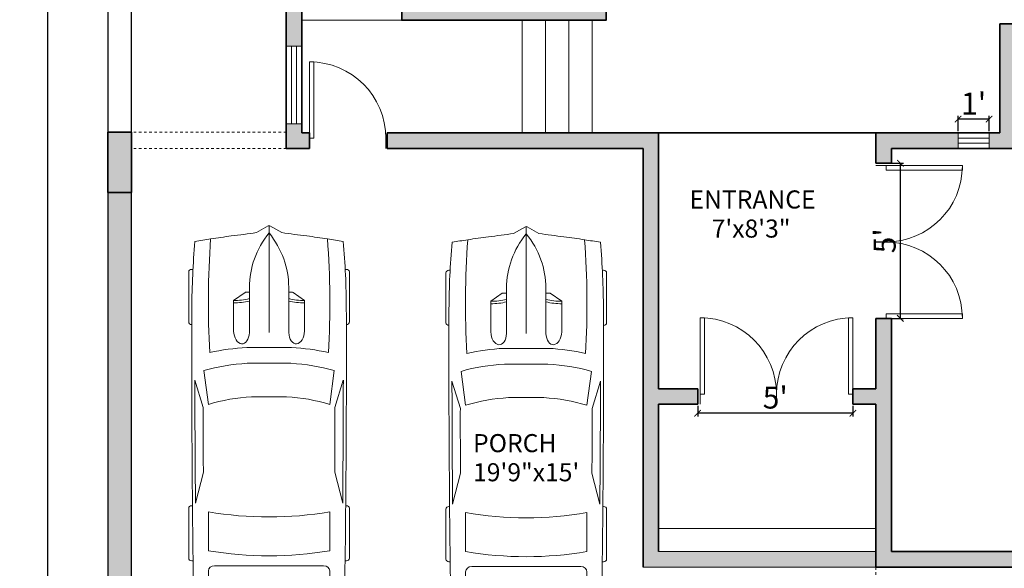
# Model space of a CAD drawing. Units: inches. Extents: x 3799 to 20199, y 1682 to 8087.
# Tile 7 of 30: x 10985 to 11366, y 2325 to 2537. Entities that reach past the tile are written whole.
import ezdxf

# ---------------------------------------------------------------- set-up
doc = ezdxf.new("R2010")
doc.units = ezdxf.units.IN
doc.linetypes.add('JIS_02_1.0', pattern=[2, 1, -1])
for name, color, linetype, lineweight in [('A-ANNO-DIMS', 2, 'Continuous', 18), ('A-AREA-IDEN', 7, 'Continuous', 18), ('A-COLS', 251, 'Continuous', 35), ('A-DOOR', 3, 'Continuous', 18), ('A-FLOR-STRS', 41, 'Continuous', 18), ('A-GLAZ', 152, 'Continuous', 18), ('A-SITE-OVHD', 8, 'JIS_02_1.0', 18), ('A-SITE-VEHC', 8, 'Continuous', 13), ('A-WALL', 7, 'Continuous', 35), ('A-WALL-PATT', 252, 'Continuous', 13), ('C-PROP', 7, 'Continuous', 25), ('L-PLNT-PATT', 94, 'Continuous', 13)]:
    doc.layers.add(name, color=color, linetype=linetype, lineweight=lineweight)
doc.styles.get("Standard").update_dxf_attribs({"font": 'arial.ttf'})
doc.dimstyles.new('ISO-25', dxfattribs={"dimtxt": 8.5, "dimasz": 2.5, "dimexe": 1.25, "dimexo": 0.625, "dimtad": 1, "dimdec": 0, "dimlunit": 3, "dimtxsty": 'Standard', "dimblk": 'ARCHTICK', "dimcen": 2.5, "dimadec": 0, "dimazin": 0, "dimtfac": 1, "dimtdec": 0, "dimtmove": 0, "dimatfit": 3, "dimfxl": 1, "dimarcsym": 0})

# ---------------------------------------------------------------- blocks, each defined once
blk = doc.blocks.new('*U47')
for p, q in [((0, 0), (0, -100)), ((750, 0), (750, -100))]:
    blk.add_line(p, q)
blk.add_lwpolyline([(0, 0), (0, 750), (43.75, 750), (43.75, 0)], close=True)
blk.add_arc((0, 0), 750, 0, 90)
blk = doc.blocks.new('_ArchTick')
at = {"color": 0, "linetype": 'ByBlock', "const_width": 0.15}
blk.add_lwpolyline([(-0.5, -0.5), (0.5, 0.5)], dxfattribs=at)
blk = doc.blocks.new('*D75')
at = {"layer": 'A-ANNO-DIMS', "color": 0, "lineweight": -2, "transparency": 16777216}
for p, q in [((11347.67, 2493.7), (11347.67, 2499.67)), ((11359.67, 2498.42), (11347.67, 2498.42)), ((11359.67, 2493.7), (11359.67, 2499.67))]:
    blk.add_line(p, q, dxfattribs=at)
at = {"layer": 'Defpoints', "color": 0, "transparency": 16777216}
for p in [(11347.67, 2498.42), (11347.67, 2493.07), (11359.67, 2493.07)]:
    blk.add_point(p, dxfattribs=at)
at = {"layer": 'A-ANNO-DIMS', "color": 0, "lineweight": -2, "transparency": 16777216, "xscale": 2.5, "yscale": 2.5, "zscale": 2.5, "rotation": 180}
blk.add_blockref('_ArchTick', (11347.67, 2498.42), dxfattribs=at)
at = {"layer": 'A-ANNO-DIMS', "color": 0, "lineweight": -2, "transparency": 16777216, "xscale": 2.5, "yscale": 2.5, "zscale": 2.5}
blk.add_blockref('_ArchTick', (11359.67, 2498.42), dxfattribs=at)
at = {"layer": 'A-ANNO-DIMS', "color": 0, "transparency": 16777216, "insert": (11353.67, 2503.31), "char_height": 8.5, "attachment_point": 5}
blk.add_mtext("1'", dxfattribs=at)
blk = doc.blocks.new('*D77')
at = {"layer": 'A-ANNO-DIMS', "color": 0, "lineweight": -2, "transparency": 16777216}
for p, q in [((11018.23, 3204.07), (10994.27, 3204.07)), ((10995.52, 3204.07), (10995.52, 2124.07)), ((11018.23, 2124.07), (10994.27, 2124.07))]:
    blk.add_line(p, q, dxfattribs=at)
at = {"layer": 'Defpoints', "color": 0, "transparency": 16777216}
for p in [(11018.85, 3204.07), (10995.52, 2124.07), (11018.85, 2124.07)]:
    blk.add_point(p, dxfattribs=at)
at = {"layer": 'A-ANNO-DIMS', "color": 0, "lineweight": -2, "transparency": 16777216, "xscale": 2.5, "yscale": 2.5, "zscale": 2.5}
for p, rotation in [((10995.52, 3204.07), 90), ((10995.52, 2124.07), 270)]:
    blk.add_blockref('_ArchTick', p, dxfattribs=dict(at, rotation=rotation))
at = {"layer": 'A-ANNO-DIMS', "color": 0, "transparency": 16777216, "insert": (10990.56, 2664.07), "char_height": 8.5, "attachment_point": 5, "rotation": 90}
blk.add_mtext("90'", dxfattribs=at)
blk = doc.blocks.new('*D81')
at = {"layer": 'A-ANNO-DIMS', "color": 0, "lineweight": -2, "transparency": 16777216}
for p, q in [((11316.48, 2481.32), (11326.57, 2481.32)), ((11325.32, 2481.32), (11325.32, 2421.32)), ((11316.48, 2421.32), (11326.57, 2421.32))]:
    blk.add_line(p, q, dxfattribs=at)
at = {"layer": 'Defpoints', "color": 0, "transparency": 16777216}
for p in [(11315.85, 2481.32), (11315.85, 2421.32), (11325.32, 2421.32)]:
    blk.add_point(p, dxfattribs=at)
at = {"layer": 'A-ANNO-DIMS', "color": 0, "lineweight": -2, "transparency": 16777216, "xscale": 2.5, "yscale": 2.5, "zscale": 2.5}
for p, rotation in [((11325.32, 2481.32), 90), ((11325.32, 2421.32), 270)]:
    blk.add_blockref('_ArchTick', p, dxfattribs=dict(at, rotation=rotation))
at = {"layer": 'A-ANNO-DIMS', "color": 0, "transparency": 16777216, "insert": (11320.37, 2451.32), "char_height": 8.5, "attachment_point": 5, "rotation": 90}
blk.add_mtext("5'", dxfattribs=at)
blk = doc.blocks.new('*D82')
at = {"layer": 'A-ANNO-DIMS', "color": 0, "lineweight": -2, "transparency": 16777216}
for p, q in [((11246.96, 2387.45), (11246.96, 2383.36)), ((11306.96, 2387.45), (11306.96, 2383.36)), ((11306.96, 2384.61), (11246.96, 2384.61))]:
    blk.add_line(p, q, dxfattribs=at)
at = {"layer": 'Defpoints', "color": 0, "transparency": 16777216}
for p in [(11246.96, 2388.07), (11306.96, 2388.07), (11246.96, 2384.61)]:
    blk.add_point(p, dxfattribs=at)
at = {"layer": 'A-ANNO-DIMS', "color": 0, "lineweight": -2, "transparency": 16777216, "xscale": 2.5, "yscale": 2.5, "zscale": 2.5, "rotation": 180}
blk.add_blockref('_ArchTick', (11246.96, 2384.61), dxfattribs=at)
at = {"layer": 'A-ANNO-DIMS', "color": 0, "lineweight": -2, "transparency": 16777216, "xscale": 2.5, "yscale": 2.5, "zscale": 2.5}
blk.add_blockref('_ArchTick', (11306.96, 2384.61), dxfattribs=at)
at = {"layer": 'A-ANNO-DIMS', "color": 0, "transparency": 16777216, "insert": (11276.96, 2389.56), "char_height": 8.5, "attachment_point": 5}
blk.add_mtext("5'", dxfattribs=at)
blk = doc.blocks.new('*U92')
for p, q in [((46.55, 38.89), (22.35, 38.89)), ((136.7, 38.89), (160.9, 38.89)), ((21.1, 37.41), (21.1, 36.83)), ((47.8, 37.39), (47.8, 37.41)), ((87.99, 31.87), (74.76, 35.92)), ((134.31, 35.6), (119.29, 31.78)), ((135.45, 37.07), (135.45, 37.41)), ((162.15, 37.41), (162.15, 36.77)), ((186.47, -33.5), (186.47, 33.5)), ((70.03, 31.54), (86.41, 29.35)), ((138.42, 29.35), (157.25, 29.35)), ((186.47, 29.35), (167.01, 29.35)), ((188.4, -32.76), (188.4, 32.76)), ((164.52, 26.39), (164.52, -26.39)), ((32.27, 11.63), (36.13, 17.17)), ((36.13, 17.17), (50.94, 17.17)), ((32.12, 9.51), (32.12, 11.15)), ((58.92, -10.77), (58.92, 10.77)), ((66.55, -10.53), (66.55, 10.53)), ((186.47, -10.53), (186.47, 10.53)), ((3.27, 6.13), (0.1, 0.41)), ((29.77, 9.51), (51.68, 9.51)), ((82.74, 8.5), (82.74, -8.5)), ((0, 0), (51.68, 0)), ((0.1, -0.41), (3.27, -6.13)), ((29.77, -9.51), (51.68, -9.51)), ((32.12, -9.51), (32.12, -11.15)), ((32.27, -11.63), (36.13, -17.17)), ((36.13, -17.17), (50.94, -17.17)), ((86.41, -29.35), (70.03, -31.54)), ((87.99, -31.87), (74.76, -35.92)), ((134.31, -35.6), (119.29, -31.78)), ((157.25, -29.35), (138.42, -29.35)), ((167.01, -29.35), (186.47, -29.35)), ((21.1, -37.41), (21.1, -36.83)), ((47.8, -37.39), (47.8, -37.41)), ((135.45, -37.07), (135.45, -37.41)), ((162.15, -37.41), (162.15, -36.77)), ((46.55, -38.89), (22.35, -38.89)), ((136.7, -38.89), (160.9, -38.89))]:
    blk.add_line(p, q)
for centre, major_axis, ratio, start_param, end_param in [((22.35, 37.41), (0, -1.48), 0.842304, 3.141593, 4.712389), ((46.55, 37.41), (0, 1.48), 0.842304, -1.570796, 0), ((136.7, 37.41), (0, -1.48), 0.842304, 3.141593, 4.712389), ((160.9, 37.41), (0, 1.48), 0.842304, -1.570796, 0), ((266.03, -27.52), (0, 313.31), 0.842304, 1.367076, 1.39176), ((41.19, -490.86), (0, 528.23), 0.842304, 0.00281, 0.075598), ((64.48, -10555.62), (0, 10593.03), 0.842304, -0.013397, 0.002797), ((64.48, -10555.62), (0, -10591.55), 0.842304, 3.133765, 3.140441), ((180.63, 35.84), (0, 2.22), 0.842304, -0.013017, 1.249894), ((64.48, -10556.36), (0, 10595.31), 0.842304, -0.013397, -0.013017), ((183.98, 33.5), (0, -2.96), 0.842304, 1.570796, 3.128196), ((183.98, 32.76), (0, -5.25), 0.842304, 1.570796, 3.128196), ((37.47, -593.96), (0, -623.33), 0.842304, 3.096046, 3.200911), ((134.4, 5.39), (0, -89.78), 0.842304, 4.449482, 4.652344), ((135.29, 5.39), (0, 81.77), 0.842304, 1.245306, 1.50788), ((149.6, 2.8), (0, -79.58), 0.842304, 4.372215, 4.640744), ((95.79, -3666.35), (0, -3698.24), 0.842304, 3.134049, 3.144098), ((17.08, 0), (0, 147.02), 0.842304, 4.511394, 4.913384), ((35.91, 0), (0, 147.02), 0.842304, 4.511394, 4.913384), ((167.01, 26.39), (0, 2.96), 0.842304, 0, 1.570796), ((259.18, -27.52), (0, -305.3), 0.842304, 4.528606, 4.561838), ((-204.49, 52.4), (0, -250.96), 0.842304, 1.385369, 1.434372), ((13.04, 17.01), (0, 27.42), 0.842304, 4.435146, 4.718221), ((14.2, 17.01), (0, 27.42), 0.842304, 4.435146, 4.718221), ((50.79, 13.34), (6.34, -0.36), 0.603834, -1.395552, 1.581315), ((32.75, 11.15), (0, 0.74), 0.842304, 0.879714, 1.570796), ((29.77, -46.66), (0, 56.17), 0.842304, 0, 0.590319), ((0.62, 0), (0, -0.74), 0.842304, 4.131459, 5.293319), ((29.77, 46.66), (0, 56.17), 0.842304, 2.551274, 3.141593), ((-204.49, -52.4), (0, 250.96), 0.842304, -1.434372, -1.385369), ((13.04, -17.01), (0, -27.42), 0.842304, 1.564964, 1.848039), ((14.2, -17.01), (0, -27.42), 0.842304, 1.564964, 1.848039), ((149.6, -2.8), (0, -79.58), 0.842304, -1.499151, -1.230623), ((32.75, -11.15), (0, -0.74), 0.842304, 4.712389, 5.403472), ((134.4, -5.39), (0, -89.78), 0.842304, -1.510751, -1.307889), ((135.29, -5.39), (0, -81.77), 0.842304, -1.50788, -1.245306), ((259.18, 27.52), (0, 305.3), 0.842304, 1.721348, 1.754579), ((266.03, 27.52), (0, 313.31), 0.842304, 1.749832, 1.774517), ((37.47, 593.96), (0, -623.33), 0.842304, -0.059319, 0.045547), ((167.01, -26.39), (0, -2.96), 0.842304, 4.712389, 6.283185), ((95.79, 3666.35), (0, -3698.24), 0.842304, -0.002505, 0.007544), ((183.98, -32.76), (0, -5.25), 0.842304, 0.013397, 1.570796), ((41.19, 490.86), (0, -528.23), 0.842304, -0.075598, -0.00281), ((22.35, -37.41), (0, 1.48), 0.842304, 1.570796, 3.141593), ((64.48, 10555.62), (0, 10593.03), 0.842304, 3.138796, 3.15499), ((46.55, -37.41), (0, -1.48), 0.842304, 0, 1.570796), ((64.48, 10555.62), (0, -10591.55), 0.842304, 0.001152, 0.007828), ((136.7, -37.41), (0, -1.48), 0.842304, -1.570796, 0), ((160.9, -37.41), (0, 1.48), 0.842304, 3.141593, 4.712389), ((180.63, -35.84), (0, -2.22), 0.842304, -1.249894, 0.013017), ((64.48, 10556.36), (0, 10595.31), 0.842304, 3.15461, 3.15499), ((183.98, -33.5), (0, 2.96), 0.842304, 3.15499, 4.712389)]:
    blk.add_ellipse(centre, major_axis=major_axis, ratio=ratio, start_param=start_param, end_param=end_param)
at = {"extrusion": (0, 0, -1)}
blk.add_ellipse((50.79, -13.34), major_axis=(6.34, 0.36), ratio=0.603834, start_param=-1.395552, end_param=1.581315, dxfattribs=at)

msp = doc.modelspace()

# ---------------------------------------------------------------- hatches: boundary and pattern name
at = {"layer": 'A-COLS'}
h = msp.add_hatch(color=256, dxfattribs=at)
h.dxf.hatch_style = 1
h.set_gradient(color1=(0, 0, 255), color2=(122, 175, 223))
h.paths.add_polyline_path([(11302.02, 2133.07), (11293.02, 2133.07), (11293.02, 2124.07), (11302.02, 2124.07)])
h.paths.add_polyline_path([(11027.85, 2133.07), (11018.85, 2133.07), (11018.85, 2124.07), (11027.85, 2124.07)])
h.paths.add_polyline_path([(11027.85, 2324.17), (11018.85, 2324.17), (11018.85, 2300.82), (11027.85, 2300.82)])
h.paths.add_polyline_path([(11027.85, 2493.31), (11018.85, 2493.31), (11018.85, 2469.95), (11027.85, 2469.95)])
at = {"layer": 'A-WALL-PATT'}
h = msp.add_hatch(color=256, dxfattribs=at)
h.dxf.hatch_style = 1
h.paths.add_polyline_path([(11549.85, 2537.07), (11543.85, 2537.07), (11543.85, 2493.07), (11500.92, 2493.07), (11500.92, 2487.07), (11543.85, 2487.07), (11543.85, 2331.07), (11512.59, 2331.07), (11512.59, 2325.07), (11549.85, 2325.07)])
h.paths.add_polyline_path([(11404.92, 2493.07), (11369.85, 2493.07), (11369.85, 2535.29), (11363.85, 2535.29), (11363.85, 2493.07), (11359.67, 2493.07), (11359.67, 2487.07), (11404.92, 2487.07)])
h.paths.add_polyline_path([(11347.67, 2493.07), (11315.85, 2493.07), (11315.85, 2481.32), (11321.85, 2481.32), (11321.85, 2487.07), (11347.67, 2487.07)])
h.paths.add_polyline_path([(11246.96, 2394.07), (11231.85, 2394.07), (11231.85, 2493.07), (11126.81, 2493.07), (11126.81, 2487.07), (11225.85, 2487.07), (11225.85, 2325.07), (11315.85, 2325.07), (11315.85, 2331.07), (11231.85, 2331.07), (11231.85, 2388.07), (11246.96, 2388.07)])
h.paths.add_polyline_path([(11368.59, 2331.07), (11321.85, 2331.07), (11321.85, 2421.32), (11319.79, 2421.32), (11315.85, 2421.32), (11315.85, 2394.07), (11306.96, 2394.07), (11306.96, 2392.01), (11306.96, 2388.07), (11315.85, 2388.07), (11315.85, 2325.07), (11368.59, 2325.07)])
h.paths.add_polyline_path([(11211.5, 2599.62), (11175.25, 2599.62), (11175.25, 2594.62), (11206.5, 2594.62), (11206.5, 2541.62), (11137.5, 2541.62), (11137.5, 2594.62), (11145.25, 2594.62), (11145.25, 2599.62), (11132.5, 2599.62), (11132.5, 2536.62), (11211.5, 2536.62)], flags=17)
h.paths.add_polyline_path([(11278.96, 2650.07), (11117.85, 2650.07), (11117.85, 2668.07), (11111.85, 2668.07), (11111.85, 2650.07), (11087.85, 2650.07), (11087.85, 2526.57), (11093.85, 2526.57), (11093.85, 2644.07), (11278.96, 2644.07)])
h.paths.add_polyline_path([(11096.81, 2491.01), (11096.81, 2493.07), (11093.85, 2493.07), (11093.85, 2496.57), (11087.85, 2496.57), (11087.85, 2487.07), (11096.81, 2487.07)])
h.paths.add_polyline_path([(11445.85, 3087.71), (11439.85, 3087.71), (11439.85, 2949.07), (11343.85, 2949.07), (11343.85, 2929.61), (11315.6, 2929.61), (11315.6, 2923.61), (11343.85, 2923.61), (11343.85, 2840.12), (11349.85, 2840.12), (11349.85, 2943.07), (11507.11, 2943.07), (11507.11, 2949.07), (11445.85, 2949.07), (11445.85, 3015.07), (11543.85, 3015.07), (11543.85, 2992.92), (11549.85, 2992.92), (11549.85, 3108.28), (11543.85, 3108.28), (11543.85, 3021.07), (11515.89, 3021.07), (11515.89, 3049.36), (11511.89, 3049.36), (11511.89, 3021.07), (11445.85, 3021.07)])
h.paths.add_polyline_path([(11549.85, 3135.07), (11408.12, 3135.07), (11408.12, 3129.07), (11439.85, 3129.07), (11439.85, 3117.71), (11443.79, 3117.71), (11445.85, 3117.71), (11445.85, 3129.07), (11504.47, 3129.07), (11504.47, 3099.65), (11508.47, 3099.65), (11508.47, 3129.07), (11543.85, 3129.07), (11543.85, 3126.28), (11549.85, 3126.28)])
h.paths.add_polyline_path([(11324.12, 3135.07), (11087.85, 3135.07), (11087.85, 3083.46), (11093.85, 3083.46), (11093.85, 3129.07), (11265.85, 3129.07), (11265.85, 3050.07), (11240.75, 3050.07), (11240.75, 3044.07), (11265.85, 3044.07), (11265.85, 2895.64), (11271.85, 2895.64), (11271.85, 2923.61), (11279.6, 2923.61), (11279.6, 2929.61), (11271.85, 2929.61), (11271.85, 3129.07), (11324.12, 3129.07)])
h.paths.add_polyline_path([(11210.75, 3050.07), (11133.85, 3050.07), (11133.85, 3088.63), (11129.85, 3088.54), (11129.85, 3050.07), (11093.85, 3050.07), (11093.85, 3059.46), (11087.85, 3059.46), (11087.85, 3030.25), (11093.85, 3030.25), (11093.85, 3044.07), (11210.75, 3044.07)], flags=17)
h.paths.add_polyline_path([(11093.85, 2982.25), (11087.85, 2982.25), (11087.85, 2913.95), (11093.85, 2913.95)], flags=17)
h.paths.add_polyline_path([(11271.85, 2859.64), (11265.85, 2859.64), (11265.85, 2854.07), (11093.85, 2854.07), (11093.85, 2865.95), (11087.85, 2865.95), (11087.85, 2848.07), (11111.85, 2848.07), (11111.85, 2812.07), (11117.85, 2812.07), (11117.85, 2848.07), (11271.85, 2848.07)])
h.paths.add_polyline_path([(11549.85, 2847.23), (11543.85, 2847.23), (11543.85, 2799.07), (11349.85, 2799.07), (11349.85, 2804.12), (11343.85, 2804.12), (11343.85, 2753.07), (11349.85, 2753.07), (11349.85, 2793.07), (11543.85, 2793.07), (11543.85, 2752.31), (11549.85, 2752.31)])
h.paths.add_polyline_path([(11549.85, 2692.31), (11543.85, 2692.31), (11543.85, 2650.07), (11343.85, 2650.07), (11338.96, 2650.07), (11338.96, 2644.07), (11349.85, 2644.07), (11363.85, 2644.07), (11363.85, 2608.29), (11369.85, 2608.29), (11369.85, 2644.07), (11543.85, 2644.07), (11543.85, 2621.07), (11549.85, 2621.07)])
h = msp.add_hatch(color=256, dxfattribs=at)
h.dxf.hatch_style = 1
h.paths.add_polyline_path([(11027.85, 2469.95), (11018.85, 2469.95), (11018.85, 2324.17), (11027.85, 2324.17)])
h.paths.add_polyline_path([(11027.85, 2300.82), (11018.85, 2300.82), (11018.85, 2133.07), (11027.85, 2133.07)])
at = {"layer": 'L-PLNT-PATT'}
h = msp.add_hatch(dxfattribs=at)
h.set_pattern_fill('GOST_GLASS', color=256)
h.paths.add_polyline_path([(11609.85, 2325.07), (11549.85, 2325.07), (11315.85, 2325.07), (11315.85, 2300.82), (11302.02, 2300.82), (11302.02, 2133.07), (11609.85, 2133.07)])
h.paths.add_polyline_path([(11496.55, 2144.31), (11496.62, 2144.39), (11496.58, 2144.52)], flags=16)
h.paths.add_polyline_path([(11491.91, 2145.12), (11493.01, 2143.36), (11494.28, 2143.99), (11494.28, 2144.01), (11494.36, 2143.39), (11494.73, 2142.84), (11494.91, 2142.94), (11495.46, 2143.67), (11495.33, 2142.52), (11496.19, 2140.15), (11495.75, 2139.78), (11494.7, 2136.83), (11492.98, 2136.07), (11493.22, 2135.99), (11492.8, 2135.99), (11491.54, 2136.62), (11490.91, 2137.68), (11490.07, 2138.1), (11489.64, 2139.15), (11489.22, 2141.04), (11489.22, 2142.73), (11489.64, 2143.71), (11490.07, 2143.57), (11491.02, 2144.77), (11491.12, 2144.24), (11491.46, 2143.95), (11491.73, 2144.28)], flags=16)
h.paths.add_polyline_path([(11491.31, 2142.42), (11493.01, 2140.83), (11492.8, 2138.94), (11491.96, 2137.47), (11490.91, 2141.04), (11491.77, 2141.99), (11490.77, 2142.92), (11491.35, 2143.4)], flags=0)
h.paths.add_polyline_path([(11455.55, 2140.87), (11453.52, 2140.87), (11451.69, 2140.04), (11455.54, 2140.52, 0.011687)], flags=16)
h.paths.add_polyline_path([(11451.82, 2137.03), (11451.82, 2136.94), (11451.92, 2136.93)], flags=16)
h.paths.add_polyline_path([(11447.97, 2140.87), (11447.97, 2135.62), (11447.21, 2136.28), (11446.7, 2139.6), (11446.1, 2139), (11446.11, 2136.84), (11446.26, 2136.47), (11446.11, 2136.28), (11446.12, 2134.9), (11445.36, 2134.39), (11445.25, 2135.18), (11446.11, 2136.28), (11446.1, 2138.85), (11445.88, 2138.78), (11443.88, 2136.78), (11442.77, 2136.56), (11443.44, 2138.06), (11441.62, 2137.52), (11442.08, 2138.6), (11442.26, 2138.61), (11442, 2138.42), (11441.62, 2137.52), (11445.88, 2138.78), (11447.97, 2140.87), (11447.97, 2143.39), (11445.18, 2146.18), (11445.72, 2147.71), (11447.97, 2146.55), (11447.97, 2148.2), (11448.27, 2147.82), (11448.02, 2146.98), (11450.07, 2142.97)], flags=16)
h.paths.add_polyline_path([(11551.41, 2140.65, -1), (11536.26, 2140.65, -1)])
h.paths.add_polyline_path([(11547.68, 2136.8), (11547.69, 2136.71), (11547.78, 2136.7)], flags=16)
h.paths.add_polyline_path([(11541.05, 2145.95), (11541.58, 2147.48), (11542.26, 2147.14), (11542.27, 2144.73)], flags=16)
h.paths.add_polyline_path([(11541.96, 2138.78), (11541.97, 2136.62), (11542.12, 2136.24), (11541.97, 2136.06), (11541.98, 2134.67), (11541.23, 2134.17), (11541.11, 2134.95), (11541.97, 2136.06), (11541.96, 2138.62), (11541.74, 2138.56), (11539.74, 2136.56), (11538.63, 2136.33), (11539.3, 2137.83), (11537.48, 2137.29), (11537.94, 2138.37), (11538.12, 2138.38), (11541.25, 2140.65), (11543.83, 2140.65)], flags=16)
h.paths.add_polyline_path([(11584.29, 2268.01), (11584.1, 2268.75), (11584.25, 2269.39), (11584.02, 2270.08), (11583.56, 2270.33), (11584.06, 2270.63), (11584.18, 2271.22), (11584.1, 2271.81), (11584.48, 2272.21), (11584.83, 2272.85), (11584.45, 2273.49), (11583.87, 2273.79), (11584.72, 2273.79), (11585.41, 2273.89), (11585.79, 2274.33), (11585.79, 2274.73), (11586.3, 2275.17), (11587.03, 2275.22), (11587.76, 2275.66), (11588.26, 2275.62), (11588.72, 2275.91), (11589.22, 2275.66), (11589.53, 2276.8), (11589.69, 2275.91), (11590.23, 2275.81), (11590.92, 2276.11), (11591.46, 2276.26), (11592.73, 2275.22), (11593.19, 2274.92), (11593.58, 2275.12), (11594.35, 2274.87), (11594.31, 2274.38), (11594.43, 2274.03), (11595.08, 2273.34), (11595.47, 2272.9), (11595.54, 2271.76), (11595.89, 2271.47), (11596.85, 2271.47), (11597.55, 2271.52), (11596.78, 2271.22), (11596.08, 2270.87), (11595.93, 2270.43), (11596.04, 2269.79), (11595.85, 2269.58), (11596.25, 2269.39), (11596.63, 2270.81), (11596.82, 2269.7), (11597.5, 2269.57), (11598.36, 2269.94), (11599.04, 2270.13), (11600.63, 2268.83), (11601.21, 2268.46), (11601.77, 2268.75), (11601.65, 2268.95), (11601.29, 2269.14), (11601.82, 2269.14), (11602.25, 2269.2), (11602.49, 2269.48), (11602.49, 2269.72), (11602.81, 2270), (11603.26, 2270.03), (11603.72, 2270.31), (11604.04, 2270.28), (11604.32, 2270.46), (11604.64, 2270.31), (11604.83, 2271.02), (11604.93, 2270.46), (11605.26, 2270.4), (11605.7, 2270.59), (11606.03, 2270.68), (11606.83, 2270.03), (11607.12, 2269.85), (11607.36, 2269.97), (11607.84, 2269.82), (11607.82, 2269.51), (11607.89, 2269.29), (11608.3, 2268.86), (11608.54, 2268.58), (11608.59, 2267.87), (11608.8, 2267.68), (11609.4, 2267.68), (11609.84, 2267.72), (11609.36, 2267.53), (11608.92, 2267.31), (11608.83, 2267.04), (11608.9, 2266.64), (11608.73, 2266.45), (11608.63, 2265.68), (11608.75, 2265.52), (11608.66, 2265.46), (11608.44, 2265.04), (11608.03, 2264.97), (11608.39, 2264.54), (11607.96, 2264.63), (11607.84, 2264.57), (11607.82, 2264.32), (11607.45, 2263.98), (11607.26, 2263.7), (11606.85, 2263.64), (11606.54, 2263.39), (11606.01, 2263.24), (11605.65, 2263.27), (11605.31, 2263.15), (11605.21, 2263.02), (11605.12, 2262.28), (11604.9, 2263.02), (11604.71, 2263.08), (11604.63, 2262.84), (11604.77, 2262.04), (11604.43, 2261.67), (11604.24, 2260.13), (11604.48, 2259.82), (11604.29, 2259.69), (11604, 2259.14), (11603.76, 2258.83), (11603.04, 2258.71), (11603.76, 2257.84), (11602.89, 2258.03), (11602.65, 2257.9), (11602.6, 2257.41), (11601.88, 2256.73), (11601.49, 2256.17), (11600.68, 2256.05), (11600.05, 2255.56), (11598.99, 2255.25), (11598.27, 2255.31), (11597.59, 2255.06), (11597.4, 2254.82), (11597.21, 2253.33), (11596.77, 2254.82), (11595.19, 2255.25), (11594.51, 2255.31), (11593.79, 2255.87), (11593.21, 2256.48), (11592.73, 2256.61), (11592.1, 2256.17), (11591.48, 2255.56), (11591.81, 2256.36), (11591.91, 2257.47), (11591.53, 2257.96), (11590.75, 2258.34), (11590.75, 2258.95), (11590.61, 2259.45), (11590.08, 2259.82), (11589.84, 2260.74), (11590.03, 2261.55), (11589.74, 2262.41), (11589.17, 2262.72), (11589.79, 2263.09), (11589.84, 2263.34), (11589.65, 2264.01), (11588.38, 2264.35), (11587.84, 2264.4), (11587.26, 2264.85), (11586.8, 2265.34), (11586.41, 2265.44), (11585.91, 2265.09), (11585.41, 2264.6), (11585.68, 2265.24), (11585.76, 2266.13), (11585.45, 2266.53), (11584.83, 2266.82), (11584.83, 2267.32), (11584.72, 2267.71)], flags=16)
h.paths.add_polyline_path([(11589.76, 2270.08), (11589.88, 2270.23), (11589.99, 2270.08)], flags=0)
h.paths.add_polyline_path([(11596.92, 2262.41), (11597.06, 2262.6), (11597.21, 2262.41)], flags=0)
h.paths.add_polyline_path([(11607.36, 2210.31), (11607.43, 2210.39), (11607.39, 2210.52)], flags=16)
h.paths.add_polyline_path([(11600.87, 2204.1), (11600.45, 2205.15), (11600.03, 2207.04), (11600.03, 2208.73), (11600.45, 2209.71), (11600.87, 2209.57), (11601.83, 2210.77), (11601.93, 2210.24), (11602.27, 2209.95), (11602.54, 2210.28), (11602.72, 2211.12), (11603.82, 2209.36), (11605.09, 2209.99), (11605.09, 2210), (11605.17, 2209.39), (11605.54, 2208.84), (11605.72, 2208.94), (11606.27, 2209.67), (11606.14, 2208.52), (11607, 2206.15), (11606.56, 2205.78), (11605.51, 2202.83), (11603.79, 2202.07), (11604.03, 2201.99), (11603.61, 2201.99), (11602.35, 2202.62), (11601.72, 2203.68)], flags=16)
h.paths.add_polyline_path([(11601.72, 2207.04), (11602.58, 2207.99), (11601.57, 2208.92), (11602.16, 2209.4), (11602.12, 2208.42), (11603.82, 2206.83), (11603.61, 2204.94), (11602.77, 2203.47)], flags=0)
h.paths.add_polyline_path([(11399.57, 2144.02), (11399.64, 2144.1), (11399.6, 2144.23)], flags=16)
h.paths.add_polyline_path([(11398.77, 2139.49), (11397.71, 2136.54), (11396, 2135.78), (11396.24, 2135.7), (11395.82, 2135.7), (11394.55, 2136.33), (11393.92, 2137.38), (11393.08, 2137.81), (11392.66, 2138.86), (11392.24, 2140.75), (11392.24, 2142.44), (11392.66, 2143.42), (11393.08, 2143.28), (11394.04, 2144.48), (11394.14, 2143.95), (11394.47, 2143.66), (11394.74, 2143.99), (11394.93, 2144.83), (11396.03, 2143.07), (11397.29, 2143.7), (11397.3, 2143.71), (11397.37, 2143.1), (11397.75, 2142.55), (11397.92, 2142.65), (11398.47, 2143.38), (11398.34, 2142.23), (11399.21, 2139.86)], flags=16)
h.paths.add_polyline_path([(11609.04, 2180.55, -1), (11593.89, 2180.55, -1)], flags=16)
h.paths.add_polyline_path([(11605.31, 2176.71), (11605.32, 2176.61), (11605.41, 2176.6)], flags=0)
h.paths.add_polyline_path([(11601.47, 2180.55), (11601.47, 2183.07), (11598.68, 2185.85), (11599.22, 2187.38), (11601.47, 2186.23), (11601.47, 2187.88), (11601.76, 2187.5), (11601.52, 2186.66), (11603.57, 2182.65), (11601.47, 2180.55), (11601.47, 2175.3), (11600.7, 2175.96), (11600.2, 2179.28), (11599.6, 2178.68), (11599.61, 2176.52), (11599.75, 2176.15), (11599.61, 2175.96), (11599.61, 2174.57), (11598.86, 2174.07), (11598.74, 2174.85), (11599.61, 2175.96), (11599.6, 2178.53), (11599.38, 2178.46), (11597.38, 2176.46), (11596.27, 2176.23), (11596.94, 2177.74), (11595.11, 2177.19), (11595.58, 2178.28), (11595.76, 2178.28), (11598.89, 2180.55)], flags=0)
h.paths.add_polyline_path([(11394.33, 2142.12), (11396.03, 2140.54), (11395.82, 2138.65), (11394.98, 2137.17), (11393.92, 2140.75), (11394.78, 2141.7), (11393.78, 2142.63), (11394.36, 2143.11)], flags=0)
h.paths.add_polyline_path([(11604.97, 2266.82), (11605.05, 2266.91), (11605.12, 2266.82)], flags=0)
h.paths.add_polyline_path([(11593.36, 2312.93, -1), (11608.51, 2312.93, -1)], flags=16)
h.paths.add_polyline_path([(11604.78, 2309.09), (11604.79, 2309), (11604.88, 2308.99)], flags=0)
h.paths.add_polyline_path([(11596.4, 2310.12), (11594.58, 2309.58), (11595.04, 2310.66), (11595.22, 2310.66), (11598.35, 2312.93), (11600.93, 2312.93), (11600.93, 2315.45), (11598.15, 2318.23), (11598.68, 2319.77), (11600.93, 2318.61), (11600.93, 2320.26), (11601.23, 2319.88), (11600.99, 2319.04), (11603.03, 2315.03), (11600.93, 2312.93), (11600.93, 2307.68), (11600.17, 2308.34), (11599.66, 2311.66), (11599.06, 2311.06), (11599.07, 2308.9), (11599.22, 2308.53), (11599.07, 2308.34), (11599.08, 2306.96), (11598.33, 2306.45), (11598.21, 2307.24), (11599.07, 2308.34), (11599.06, 2310.91), (11598.84, 2310.84), (11596.84, 2308.84), (11595.73, 2308.62)], flags=0)
h.paths.add_polyline_path([(11605.66, 2145.72), (11605.73, 2145.8), (11605.69, 2145.93)], flags=16)
h.paths.add_polyline_path([(11598.75, 2140.56), (11598.33, 2142.46), (11598.33, 2144.14), (11598.75, 2145.12), (11599.17, 2144.98), (11600.13, 2146.18), (11600.23, 2145.66), (11600.56, 2145.36), (11600.83, 2145.69), (11601.02, 2146.53), (11602.12, 2144.77), (11603.38, 2145.4), (11603.39, 2145.42), (11603.46, 2144.81), (11603.84, 2144.25), (11604.02, 2144.35), (11604.56, 2145.08), (11604.44, 2143.93), (11605.3, 2141.56), (11604.86, 2141.19), (11603.8, 2138.25), (11602.09, 2137.48), (11602.33, 2137.4), (11601.91, 2137.4), (11600.65, 2138.04), (11600.01, 2139.09), (11599.17, 2139.51)], flags=16)
h.paths.add_polyline_path([(11600.01, 2142.46), (11600.87, 2143.4), (11599.87, 2144.33), (11600.45, 2144.81), (11600.42, 2143.83), (11602.12, 2142.25), (11601.91, 2140.35), (11601.07, 2138.88)], flags=0)
h.paths.add_polyline_path([(11363.83, 2141.59, -1), (11348.68, 2141.59, -1)], flags=0)
h.paths.add_polyline_path([(11360.1, 2137.75), (11360.11, 2137.66), (11360.2, 2137.65)], flags=0)
h.paths.add_polyline_path([(11356.26, 2141.59), (11356.26, 2136.34), (11355.49, 2137), (11354.98, 2140.32), (11354.38, 2139.72), (11354.39, 2137.56), (11354.54, 2137.19), (11354.39, 2137), (11354.4, 2135.62), (11353.65, 2135.11), (11353.53, 2135.9), (11354.39, 2137), (11354.38, 2139.57), (11354.17, 2139.5), (11352.16, 2137.5), (11351.05, 2137.28), (11351.73, 2138.78), (11349.9, 2138.24), (11350.36, 2139.32), (11350.54, 2139.33), (11353.68, 2141.59), (11356.26, 2141.59), (11356.26, 2144.11), (11353.47, 2146.9), (11354.01, 2148.43), (11356.26, 2147.27), (11356.26, 2148.92), (11356.55, 2148.54), (11356.31, 2147.7), (11358.35, 2143.69)], flags=0)
h.paths.add_polyline_path([(11313.11, 2243.68), (11313.18, 2243.77), (11313.14, 2243.89)], flags=16)
h.paths.add_polyline_path([(11312.31, 2239.16), (11311.26, 2236.21), (11309.55, 2235.45), (11309.79, 2235.37), (11309.37, 2235.37), (11308.1, 2236), (11307.47, 2237.05), (11306.63, 2237.47), (11306.21, 2238.53), (11305.79, 2240.42), (11305.79, 2242.11), (11306.21, 2243.09), (11306.63, 2242.95), (11307.59, 2244.15), (11307.68, 2243.62), (11308.02, 2243.32), (11308.29, 2243.65), (11308.47, 2244.5), (11309.58, 2242.74), (11310.84, 2243.37), (11310.85, 2243.38), (11310.92, 2242.77), (11311.3, 2242.22), (11311.47, 2242.32), (11312.02, 2243.05), (11311.89, 2241.9), (11312.75, 2239.53)], flags=16)
h.paths.add_polyline_path([(11308.52, 2236.84), (11307.47, 2240.42), (11308.33, 2241.37), (11307.33, 2242.3), (11307.91, 2242.78), (11307.87, 2241.79), (11309.58, 2240.21), (11309.37, 2238.32)], flags=0)
h.paths.add_polyline_path([(11302.02, 2281.94, -1), (11317.17, 2281.94, -1)])
h.paths.add_polyline_path([(11313.44, 2278.1), (11313.44, 2278), (11313.54, 2277.99)], flags=16)
h.paths.add_polyline_path([(11309.59, 2276.69), (11308.83, 2277.35), (11308.32, 2280.67), (11307.72, 2280.07), (11307.73, 2277.91), (11307.88, 2277.54), (11307.73, 2277.35), (11307.74, 2275.96), (11306.98, 2275.46), (11306.87, 2276.24), (11307.73, 2277.35), (11307.72, 2279.92), (11307.5, 2279.85), (11305.5, 2277.85), (11304.39, 2277.63), (11305.06, 2279.13), (11303.24, 2278.58), (11303.7, 2279.67), (11303.88, 2279.67), (11303.62, 2279.49), (11303.24, 2278.58), (11307.5, 2279.85), (11309.59, 2281.94), (11309.59, 2284.46), (11306.8, 2287.24), (11307.34, 2288.77), (11309.59, 2287.62), (11309.59, 2289.27), (11309.89, 2288.89), (11309.64, 2288.05), (11311.69, 2284.04), (11309.59, 2281.94)], flags=16)
h.paths.add_polyline_path([(11317.17, 2181.83, -1), (11302.02, 2181.83, -1)])
h.paths.add_polyline_path([(11313.44, 2177.98), (11313.44, 2177.89), (11313.54, 2177.88)], flags=16)
h.paths.add_polyline_path([(11309.59, 2181.83), (11309.59, 2176.58), (11308.83, 2177.24), (11308.32, 2180.56), (11307.72, 2179.96), (11307.73, 2177.8), (11307.88, 2177.42), (11307.73, 2177.24), (11307.74, 2175.85), (11306.98, 2175.35), (11306.87, 2176.13), (11307.73, 2177.24), (11307.72, 2179.8), (11307.5, 2179.74), (11305.5, 2177.74), (11304.39, 2177.51), (11305.06, 2179.01), (11303.24, 2178.47), (11303.7, 2179.55), (11303.88, 2179.56), (11303.62, 2179.38), (11303.24, 2178.47), (11307.5, 2179.74), (11309.59, 2181.83), (11309.59, 2184.35), (11306.8, 2187.13), (11307.34, 2188.66), (11309.59, 2187.51), (11309.59, 2189.16), (11309.89, 2188.78), (11309.64, 2187.94), (11311.69, 2183.93)], flags=16)
h.paths.add_polyline_path([(11318.27, 2141.81), (11318.34, 2141.89), (11318.3, 2142.02)], flags=16)
h.paths.add_polyline_path([(11317.47, 2137.28), (11316.41, 2134.34), (11314.7, 2133.57), (11314.94, 2133.49), (11314.52, 2133.49), (11313.26, 2134.12), (11312.62, 2135.18), (11311.78, 2135.6), (11311.36, 2136.65), (11310.94, 2138.55), (11310.94, 2140.23), (11311.36, 2141.21), (11311.78, 2141.07), (11312.74, 2142.27), (11312.84, 2141.75), (11313.17, 2141.45), (11313.44, 2141.78), (11313.63, 2142.62), (11314.73, 2140.86), (11315.99, 2141.49), (11316, 2141.51), (11316.07, 2140.9), (11316.45, 2140.34), (11316.62, 2140.44), (11317.17, 2141.17), (11317.05, 2140.02), (11317.91, 2137.65)], flags=16)
h.paths.add_polyline_path([(11314.73, 2138.34), (11314.52, 2136.44), (11313.68, 2134.97), (11312.62, 2138.55), (11313.48, 2139.49), (11312.48, 2140.42), (11313.06, 2140.9), (11313.03, 2139.92)], flags=0)
h.paths.add_polyline_path([(11454.71, 2144.33), (11450.92, 2143.82), (11447.97, 2140.87), (11455.55, 2140.87, 0.119183)], flags=16)
h.paths.add_polyline_path([(11450.07, 2142.97), (11448.02, 2146.98), (11447.97, 2147.09), (11447.97, 2146.55), (11447.97, 2140.87)], flags=0)
h.paths.add_polyline_path([(11447.97, 2143.39), (11445.18, 2146.18), (11445.72, 2147.71), (11445.88, 2148.15, 0.334379), (11440.4, 2140.87), (11447.97, 2140.87)], flags=0)
h.paths.add_polyline_path([(11447.97, 2143.39), (11447.97, 2146.55), (11447.97, 2148.45, 0.414214), (11440.4, 2140.87), (11447.97, 2140.87)], flags=16)
h.paths.add_polyline_path([(11447.97, 2138.46), (11447.97, 2135.62), (11447.97, 2133.3, 0.158969), (11452.44, 2134.75), (11450.84, 2136.28), (11451.1, 2135.2), (11450.97, 2134.44)], flags=16)
h.paths.add_polyline_path([(11348.68, 2141.59, 1), (11363.83, 2141.59, 1)], flags=16)
h.paths.add_polyline_path([(11360.1, 2137.75), (11360.28, 2135.9), (11359.13, 2137), (11358.61, 2139.24)], flags=0)
h.paths.add_polyline_path([(11362.99, 2145.05), (11359.2, 2144.54), (11356.26, 2141.59), (11361.81, 2141.59), (11363.78, 2142.49, 0.08904)], flags=0)

# ---------------------------------------------------------------- linework, layer by layer
at = {"layer": 'A-COLS'}
msp.add_lwpolyline([(11018.85, 2469.95), (11027.95, 2469.95), (11027.95, 2493.31), (11018.85, 2493.31)], close=True, dxfattribs=at)
at = {"layer": 'A-FLOR-STRS'}
for p, q in [((11132.5, 2536.62), (11093.85, 2536.62)), ((11179.12, 2536.62), (11179.12, 2493.07)), ((11188.12, 2536.62), (11188.12, 2493.07)), ((11197.12, 2536.62), (11197.12, 2493.07)), ((11206.12, 2536.62), (11206.12, 2493.07)), ((11315.85, 2340.07), (11231.85, 2340.07)), ((11315.85, 2331.07), (11231.85, 2331.07)), ((11315.85, 2325.07), (11225.85, 2325.07))]:
    msp.add_line(p, q, dxfattribs=at)
at = {"layer": 'A-GLAZ'}
for p, q in [((11093.85, 2526.57), (11087.85, 2526.57)), ((11089.85, 2526.57), (11089.85, 2496.57)), ((11091.85, 2526.57), (11091.85, 2496.57)), ((11093.85, 2496.57), (11087.85, 2496.57)), ((11347.67, 2493.07), (11347.67, 2487.07)), ((11359.67, 2491.07), (11347.67, 2491.07)), ((11359.67, 2493.07), (11359.67, 2487.07)), ((11359.67, 2489.07), (11347.67, 2489.07))]:
    msp.add_line(p, q, dxfattribs=at)
at = {"layer": 'A-SITE-OVHD'}
for p, q in [((11027.85, 2493.31), (11018.85, 2493.31)), ((11087.85, 2493.31), (11027.85, 2493.31)), ((11087.85, 2487.07), (11027.85, 2487.07)), ((11315.85, 2325.07), (11315.85, 2300.82))]:
    msp.add_line(p, q, dxfattribs=at)
at = {"layer": 'A-WALL'}
for p, q in [((11087.85, 2650.07), (11087.85, 2487.07)), ((11093.85, 2644.07), (11093.85, 2493.07)), ((11363.85, 2493.07), (11363.85, 2535.29)), ((11363.85, 2535.29), (11369.85, 2535.29)), ((11096.81, 2493.07), (11093.85, 2493.07)), ((11096.81, 2493.07), (11096.81, 2487.07)), ((11231.85, 2493.07), (11126.81, 2493.07)), ((11126.81, 2493.07), (11126.81, 2487.07)), ((11315.85, 2493.07), (11231.85, 2493.07)), ((11231.85, 2394.07), (11231.85, 2493.07)), ((11363.85, 2493.07), (11315.85, 2493.07)), ((11315.85, 2481.32), (11315.85, 2493.07)), ((11096.81, 2487.07), (11087.85, 2487.07)), ((11225.85, 2487.07), (11126.81, 2487.07)), ((11225.85, 2325.07), (11225.85, 2487.07)), ((11321.85, 2481.32), (11321.85, 2487.07)), ((11404.92, 2487.07), (11321.85, 2487.07)), ((11321.85, 2481.32), (11315.85, 2481.32)), ((11315.85, 2394.07), (11315.85, 2421.32)), ((11321.85, 2421.32), (11315.85, 2421.32)), ((11321.85, 2331.07), (11321.85, 2421.32)), ((11246.96, 2394.07), (11231.85, 2394.07)), ((11246.96, 2394.07), (11246.96, 2388.07)), ((11315.85, 2394.07), (11306.96, 2394.07)), ((11306.96, 2394.07), (11306.96, 2388.07)), ((11246.96, 2388.07), (11231.85, 2388.07)), ((11231.85, 2331.07), (11231.85, 2388.07)), ((11315.85, 2388.07), (11306.96, 2388.07)), ((11315.85, 2325.07), (11315.85, 2388.07)), ((11543.85, 2331.07), (11321.85, 2331.07)), ((11549.85, 2325.07), (11315.85, 2325.07))]:
    msp.add_line(p, q, dxfattribs=at)
msp.add_lwpolyline([(11175.25, 2599.62), (11211.5, 2599.62), (11211.5, 2536.62), (11132.5, 2536.62), (11132.5, 2599.62), (11145.25, 2599.62)], dxfattribs=at)
at = {"layer": 'C-PROP'}
for p, q in [((11018.85, 3204.07), (11018.85, 2124.07)), ((11027.85, 3195.07), (11027.85, 2133.07))]:
    msp.add_line(p, q, dxfattribs=at)

# ---------------------------------------------------------------- block references
at = {"layer": 'A-DOOR', "yscale": 0.0393700787401575, "zscale": 0.0393700787401575}
for p, xscale in [((11096.81, 2491.01), 0.0393700787401575), ((11247.9, 2392.01), 0.0393700787401575), ((11306.96, 2392.01), -0.0393700787401575)]:
    msp.add_blockref('*U47', p, dxfattribs=dict(at, xscale=xscale))
at = {"layer": 'A-DOOR', "yscale": 0.0393700787401575, "zscale": 0.0393700787401575, "rotation": 270}
for p, xscale in [((11319.79, 2480.38), 0.0393700787401575), ((11319.79, 2421.32), -0.0393700787401575)]:
    msp.add_blockref('*U47', p, dxfattribs=dict(at, xscale=xscale))
at = {"layer": 'A-SITE-VEHC', "xscale": 0.7993080490319063, "yscale": 0.7993080490319063, "zscale": 0.7993080490319063, "rotation": 270}
for p in [(11081.21, 2457.12), (11180.65, 2456.79)]:
    msp.add_blockref('*U92', p, dxfattribs=at)

# ---------------------------------------------------------------- texts
at = {"layer": 'A-AREA-IDEN'}
for s, p in [('ENTRANCE', (11243.8, 2463.8)), ('    7\'x8\'3"', (11243.8, 2452.55)), ('PORCH', (11160.09, 2369.54)), ('19\'9"x15\'', (11160.09, 2358.29))]:
    msp.add_text(s, height=7, rotation=0.0019, dxfattribs=at).set_placement(p)

# ---------------------------------------------------------------- dimensions: what is measured, and where the dimension line sits
at = {"layer": 'A-ANNO-DIMS'}
for base, p1, p2, picture, middle in [((10995.52, 2124.07), (11018.85, 3204.07), (11018.85, 2124.07), '*D77', (10990.56, 2664.07)), ((11325.32, 2421.32), (11315.85, 2481.32), (11315.85, 2421.32), '*D81', (11320.37, 2451.32))]:
    dim = msp.add_linear_dim(base=base, p1=p1, p2=p2, angle=90, dimstyle='ISO-25', override={"dimclrd": 0, "dimclre": 0, "dimclrt": 0}, dxfattribs=at)
    dim.commit()
    dim.dimension.update_dxf_attribs({"geometry": picture, "text_midpoint": middle})
for base, p1, p2, picture, middle in [((11347.67, 2498.42), (11359.67, 2493.07), (11347.67, 2493.07), '*D75', (11353.67, 2503.31)), ((11246.96, 2384.61), (11306.96, 2388.07), (11246.96, 2388.07), '*D82', (11276.96, 2389.56))]:
    dim = msp.add_linear_dim(base=base, p1=p1, p2=p2, dimstyle='ISO-25', override={"dimclrd": 0, "dimclre": 0, "dimclrt": 0}, dxfattribs=at)
    dim.commit()
    dim.dimension.update_dxf_attribs({"geometry": picture, "text_midpoint": middle})

doc.saveas('drawing.dxf')
